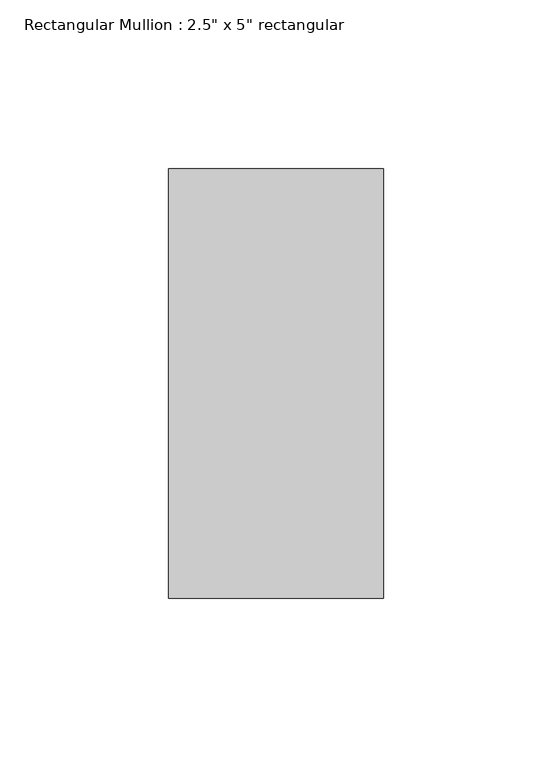
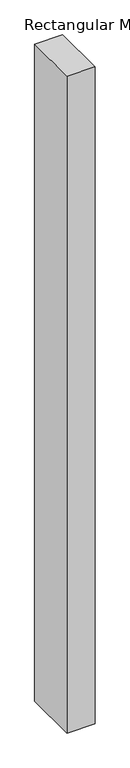
"""IFC4 building model written with IfcOpenShell, lengths in millimetres: member geometry."""

from ifc_helpers import new_model, si_unit, frame, origin, place, context, project, spatial, polyline, outline, extrude, source, transform, mapped, element, save


def member_9145ce8f(model_context):
    return source(origin(), model_context, "Body", "SweptSolid", [
        extrude(outline(polyline([(31.75, 63.5), (31.75, -63.5), (-31.75, -63.5), (-31.75, 63.5), (31.75, 63.5)])), frame((0.0, 0.0, -1576.8375758), z_axis=(0.0, 0.0, 1.0), x_axis=(1.0, 0.0, 0.0)), (0.0, 0.0, 1.0), 1576.8375758),
    ])


if __name__ == "__main__":
    model = new_model("IFC4")
    model_context = context("Model", 3, world=origin())
    ifc_project = project(units=[si_unit("LENGTHUNIT", "METRE", prefix="MILLI")], contexts=[model_context])
    site = spatial("IfcSite", under=ifc_project)
    building = spatial("IfcBuilding", under=site)
    placement = place(None, origin())
    member_shape = member_9145ce8f(model_context)
    element("IfcMember", 1, ObjectType="Rectangular Mullion : 2.5\" x 5\" rectangular", at=placement, inside=building, context=model_context, shape_type="MappedRepresentation", body=[
        mapped(member_shape, transform((0.0, 0.0, 0.0), x_axis=(1.0, 0.0, 0.0), y_axis=(0.0, 1.0, 0.0), z_axis=(0.0, 0.0, 1.0))),
    ])
    save(model, "model.ifc")

# Revit data of these elements
# Type "Rectangular Mullion : 2.5\" x 5\" rectangular"
#   built-in parameter 1007304 = 0.416667 (stored number, unit not read)
#   built-in parameter 1007301 = 0.104167 (stored number, unit not read)
#   built-in parameter 1007300 = 0.104167 (stored number, unit not read)
# Element 1 (IfcMember, "Rectangular Mullion : 2.5\" x 5\" rectangular")
#   Materials on its faces: "Aluminum"
# Materials
#   "Aluminum": class "Metal", colour RGB 247 247 247, transparency 0, Description = "Aluminum 6061", Cost = 0
